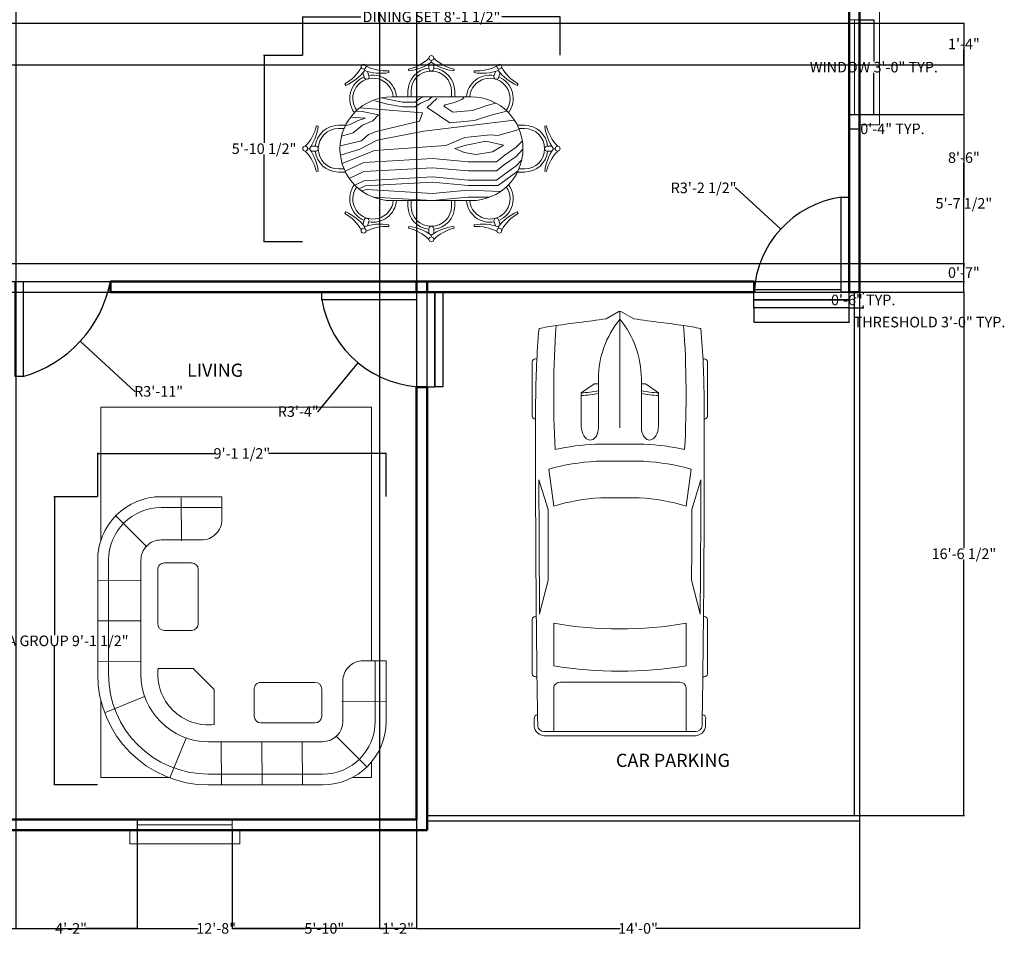
# Model space of a CAD drawing. Units: inches. Extents: x 749 to 1356, y 222 to 907.
# Tile 2 of 4: x 982 to 1356, y 222 to 570. Entities that reach past the tile are written whole.
import ezdxf

# ---------------------------------------------------------------- set-up
doc = ezdxf.new("R2010")
doc.units = ezdxf.units.IN
doc.header["$MEASUREMENT"] = 0
for name, color, linetype, lineweight in [('A-ANNO-DIMS', 30, 'Continuous', 18), ('A-AREA-IDEN', 6, 'Continuous', 25), ('A-EQPM-VEHI', 8, 'Continuous', 13), ('A-FLOR', 50, 'Continuous', 25), ('A-GLAZ', 4, 'Continuous', 20), ('A-WALL', 7, 'Continuous', 50), ('DOOR', 4, 'Continuous', 25), ('FURNITURE', 32, 'Continuous', 18)]:
    doc.layers.add(name, color=color, linetype=linetype, lineweight=lineweight)
doc.styles.get("Standard").update_dxf_attribs({"font": 'arial.ttf'})
doc.dimstyles.get("Standard").update_dxf_attribs({"dimtxt": 4, "dimasz": 0.18, "dimexe": 0.18, "dimexo": 0.0625, "dimgap": 0.09, "dimtad": 0, "dimtih": 1, "dimtoh": 1, "dimdec": 0, "dimrnd": 6, "dimzin": 0, "dimdsep": 46, "dimlunit": 3, "dimtxsty": 'Standard', "dimcen": 0.09, "dimadec": 0, "dimazin": 0, "dimtfac": 1, "dimtdec": 0, "dimtofl": 0, "dimtmove": 0, "dimatfit": 3, "dimfxl": 1, "dimtolj": 1, "dimtzin": 0, "dimarcsym": 0})

# ---------------------------------------------------------------- blocks, each defined once
blk = doc.blocks.new('ОГ56_на8персон_стол1760х1000')
for p, q in [((-54.1, 413.1), (-54.1, 412.2)), ((-713.5, 329), (-713.2, 328.1)), ((-77.6, 332.9), (-77.6, 291.9)), ((-54.1, 365), (-54.1, 348.6)), ((-30.5, 332.9), (-30.5, 291.9)), ((608.1, 329), (607.9, 328.1)), ((-713.2, 245.4), (-701.4, 206.1)), ((-699.7, 282.9), (-695.1, 267.2)), ((-668, 258.9), (-656.3, 219.5)), ((-464.6, 265.8), (-464.4, 247.7)), ((-274.5, 281.4), (-269.5, 264.1)), ((166.4, 281.4), (161.4, 264.1)), ((359.3, 265.8), (359.1, 247.7)), ((562.6, 258.9), (550.9, 219.5)), ((594.4, 282.9), (589.7, 267.2)), ((607.8, 245.4), (596.1, 206.1)), ((-887.1, 139.8), (-877.4, 124.6)), ((781.8, 139.8), (772.1, 124.6)), ((-279.1, 68.1), (-279.1, 15.3)), ((-279.1, 68.1), (-279.1, 15.3)), ((-249.1, 68.1), (-249.1, 14.5)), ((140.9, 68.1), (140.9, 14.5)), ((170.9, 68.1), (170.9, 15.3)), ((-1160.9, -264.3), (-1143.6, -269.2)), ((-947.6, -259.7), (-880.1, -259.7)), ((-126.6, -314.5), (745, -208.4)), ((842.3, -259.7), (774.8, -259.7)), ((842.3, -259.7), (774.8, -259.7)), ((1055.6, -264.3), (1038.2, -269.2)), ((-947.6, -289.7), (-894, -289.7)), ((-577.1, -401.6), (-126.6, -314.5)), ((842.3, -289.7), (788.7, -289.7)), ((-1212.4, -461.1), (-1171.4, -461.1)), ((-741, -488.6), (-577.1, -401.6)), ((1107.1, -461.1), (1066, -461.1)), ((-1292.6, -484.7), (-1291.7, -484.7)), ((-1244.5, -484.7), (-1228.1, -484.7)), ((-1212.4, -508.3), (-1171.4, -508.3)), ((-929.8, -546), (-741, -488.6)), ((1107.1, -508.3), (1066, -508.3)), ((1139.2, -484.7), (1122.8, -484.7)), ((1187.3, -484.7), (1186.3, -484.7)), ((-1160.9, -705.1), (-1143.6, -700.2)), ((-947.6, -679.7), (-894, -679.7)), ((-947.6, -709.7), (-880.1, -709.7)), ((842.3, -709.7), (774.8, -709.7)), ((842.3, -679.7), (788.7, -679.7)), ((1055.6, -705.1), (1038.2, -700.2)), ((-279.1, -1037.5), (-279.1, -984.7)), ((-279.1, -1037.5), (-279.1, -984.7)), ((-249.1, -1037.5), (-249.1, -983.9)), ((140.9, -1037.5), (140.9, -983.9)), ((170.9, -1037.5), (170.9, -984.7)), ((-887.1, -1109.2), (-877.4, -1094)), ((781.8, -1109.2), (772.1, -1094)), ((-713.2, -1214.8), (-701.4, -1175.5)), ((-668, -1228.3), (-656.3, -1188.9)), ((-464.6, -1235.1), (-464.4, -1217.1)), ((359.3, -1235.1), (359.1, -1217.1)), ((562.6, -1228.3), (550.9, -1188.9)), ((607.8, -1214.8), (596.1, -1175.5)), ((-713.5, -1298.4), (-713.2, -1297.5)), ((-699.7, -1252.3), (-695.1, -1236.6)), ((-274.5, -1250.8), (-269.5, -1233.5)), ((-77.6, -1302.3), (-77.6, -1261.3)), ((-54.1, -1334.4), (-54.1, -1318)), ((-30.5, -1302.3), (-30.5, -1261.3)), ((166.4, -1250.8), (161.4, -1233.5)), ((594.4, -1252.3), (589.7, -1236.6)), ((608.1, -1298.4), (607.9, -1297.5)), ((-54.1, -1382.5), (-54.1, -1381.6))]:
    blk.add_line(p, q)
for points in [[(-598.9, -24.3), (-476.4, -56.3), (-332.7, -82.9), (-210.2, -82.9), (-157, -45.6), (-82.5, -13.7), (-46.2, 15.3)], [(-530.7, 5.8), (-476.4, -8.4), (-332.7, -35), (-210.2, -35), (-157, 2.3), (-126.6, 15.3)], [(-433.6, 15.3), (328.3, 15.3)], [(672.4, -122), (509.9, -163.9), (362.7, -214.1), (125.3, -234.2), (-93.7, -88), (0, 0)], [(79.7, -62.3), (167.8, -40.3), (247.6, -8.4), (263.1, 15.3)], [(-932.9, -458.7), (-727.6, -408.3), (-657.4, -348), (-583.8, -317.9), (-166.7, -220.8), (-140, -140.5), (-743.6, -92.4)], [(567.6, -45.7), (481.2, -68), (342.1, -115.5), (151.7, -131.6), (66.5, -74.7), (79.7, -62.3)], [(-919.1, -365), (-807.9, -331.3), (-717.6, -257.6), (-617.2, -217.5), (-563.7, -157.2), (-720.9, -127.1), (-777.6, -121.8)], [(-883.3, -266.1), (-834.6, -252.1), (-757.7, -211.9), (-687.5, -191.8), (-830, -180)], [(793.2, -300.7), (587.2, -356.4), (515.4, -351.6), (268.7, -376.9), (85.4, -452.8), (-602.4, -503.4), (-913, -626.8)], [(822.3, -407.6), (762.6, -471.2), (653.6, -547.1), (573.6, -610.4), (301.7, -610.4), (-41.8, -578.8), (-702.3, -616.7), (-884.6, -700.6)], [(828.2, -490.2), (762.6, -560.1), (651.1, -636), (573.6, -699.3), (301.7, -699.3), (-41.8, -667.6), (-702.3, -705.6), (-843.8, -770.7)], [(816.8, -591.3), (762.6, -648.9), (658.7, -724.9), (573.6, -788.2), (301.7, -788.2), (-41.8, -756.5), (-702.3, -794.5), (-790.4, -835)], [(780.6, -697.7), (688.4, -765.1), (590.1, -838.2), (299.4, -838.2), (-42.7, -806.7), (-690, -843.9), (-750.3, -871.6)], [(609.5, -898.1), (296.3, -883.5), (-43.8, -914.8), (-673.5, -878.6), (-724.3, -891.5)], [(504.3, -952.7), (296.3, -952.7), (-43.8, -984), (-613.4, -951.3)], [(328.3, -984.7), (-433.6, -984.7)]]:
    blk.add_lwpolyline(points)
blk.add_lwpolyline([(641.8, -451.5), (534.3, -514.8), (376.2, -540.1), (262.4, -521.1), (173.9, -483.1), (281.4, -451.5), (471.1, -413.5)], close=True)
for centre in [(-54.1, 388.6), (-706.5, 305.5), (601.1, 305.5), (-1268.1, -484.7), (1162.8, -484.7), (-706.5, -1274.9), (601.1, -1274.9), (-54.1, -1358)]:
    blk.add_circle(centre, 23.6)
for centre, radius, start, end in [((-360.8, 674.3), 402.3, 282.38676, 314.74189), ((252.7, 674.3), 402.3, 225.25811, 257.61324), ((-1082, 491.8), 402.3, 298.97989, 331.33502), ((-494.1, 666.9), 402.3, 241.85124, 274.20637), ((-54.1, 68.1), 225, 96.01239, 180), ((-332.2, 740.5), 480.6, 277.49099, 305.35851), ((-54.1, 286.7), 23.6, 167.11156, 12.88844), ((224, 740.5), 480.6, 234.64149, 262.50901), ((-54.1, 68.1), 225, 0, 83.98761), ((388.8, 666.9), 402.3, 265.79363, 298.14876), ((976.7, 491.8), 402.3, 208.66498, 241.02011), ((-1073.5, 563.4), 480.6, 294.08412, 321.95164), ((-615, -1.6), 225, 112.60552, 217.31149), ((-615, -1.6), 195, 4.98125, 216.21895), ((-677.4, 207.8), 23.6, 183.7047, 29.48157), ((-540.5, 722.2), 480.6, 251.23462, 279.10214), ((-615, -1.6), 225, 4.31572, 100.58074), ((-54.1, 68.1), 195, 0, 180), ((509.6, -1.6), 225, 79.41926, 175.68428), ((509.6, -1.6), 195, 323.78105, 175.01875), ((435.1, 722.2), 480.6, 260.89786, 288.76538), ((572, 207.8), 23.6, 150.51843, 356.2953), ((968.2, 563.4), 480.6, 218.04836, 245.91588), ((509.6, -1.6), 225, 322.68851, 67.39448), ((-433.6, -484.7), 500, 90, 270), ((328.3, -484.7), 500, 270, 90), ((-1553.8, -178), 402.3, 315.25811, 347.61324), ((-1620, -206.6), 480.6, 324.64149, 352.50901), ((-947.6, -484.7), 225, 90, 173.98761), ((842.3, -484.7), 225, 6.01239, 90), ((1514.7, -206.6), 480.6, 187.49099, 215.35851), ((1448.5, -178), 402.3, 192.38676, 224.74189), ((-947.6, -484.7), 195, 90, 270), ((842.3, -484.7), 195, 270, 90), ((-1166.2, -484.7), 23.6, 257.11156, 102.88844), ((1060.8, -484.7), 23.6, 77.11156, 282.88844), ((-1553.8, -791.4), 402.3, 12.38676, 44.74189), ((-1620, -762.8), 480.6, 7.49099, 35.35851), ((-947.6, -484.7), 225, 186.01239, 270), ((842.3, -484.7), 225, 270, 353.98761), ((1514.7, -762.8), 480.6, 144.64149, 172.50901), ((1448.5, -791.4), 402.3, 135.25811, 167.61324), ((-615, -967.8), 225, 142.68851, 247.39448), ((-615, -967.8), 195, 143.78105, 355.01875), ((509.6, -967.8), 195, 184.98125, 36.21895), ((509.6, -967.8), 225, 292.60552, 37.31149), ((-615, -967.8), 225, 259.41926, 355.68428), ((-54.1, -1037.5), 225, 180, 263.98761), ((-54.1, -1037.5), 195, 180, 0), ((-54.1, -1037.5), 225, 276.01239, 0), ((509.6, -967.8), 225, 184.31572, 280.58074), ((-1082, -1461.1), 402.3, 28.66498, 61.02011), ((-1073.5, -1532.8), 480.6, 38.04836, 65.91588), ((968.2, -1532.8), 480.6, 114.08412, 141.95164), ((976.7, -1461.1), 402.3, 118.97989, 151.33502), ((-677.4, -1177.2), 23.6, 330.51843, 176.2953), ((-540.5, -1691.6), 480.6, 80.89786, 108.76538), ((435.1, -1691.6), 480.6, 71.23462, 99.10214), ((572, -1177.2), 23.6, 3.7047, 209.48157), ((-494.1, -1636.3), 402.3, 85.79363, 118.14876), ((-360.8, -1643.7), 402.3, 45.25811, 77.61324), ((-332.2, -1709.9), 480.6, 54.64149, 82.50901), ((-54.1, -1256.1), 23.6, 347.11156, 192.88844), ((224, -1709.9), 480.6, 97.49099, 125.35851), ((252.7, -1643.7), 402.3, 102.38676, 134.74189), ((388.8, -1636.3), 402.3, 61.85124, 94.20637)]:
    blk.add_arc(centre, radius, start, end)
blk = doc.blocks.new('A$C0BCD5431')
for p, q in [((2628, 4268), (940, 4268)), ((1236, 4268), (1240, 3628)), ((1836, 4268), (1840, 3628)), ((2436, 4268), (2440, 3628)), ((2628, 4108), (940, 4108)), ((2957, 3573), (3201, 4165)), ((742, 3540), (290, 3993)), ((2628, 3628), (940, 3628)), ((2542, 3373), (2545, 2855)), ((0, 3328), (0, 2432)), ((160, 3328), (160, 2431)), ((640, 3328), (640, 2730)), ((952, 3249), (952, 2849)), ((1852, 3349), (1052, 3349)), ((1952, 2849), (1952, 3249)), ((3573, 2957), (4165, 3201)), ((15, 3032), (655, 3028)), ((2545, 2855), (2855, 2545)), ((1052, 2749), (1852, 2749)), ((3628, 2628), (3628, 940)), ((4108, 2628), (4108, 940)), ((4268, 2628), (4268, 940)), ((3373, 2542), (2855, 2545)), ((0, 2432), (338, 2430)), ((4268, 2436), (3628, 2440)), ((3280, 1980), (2880, 1980)), ((2780, 1880), (2780, 1080)), ((3380, 1080), (3380, 1880)), ((4268, 1836), (3628, 1840)), ((4268, 1236), (3628, 1240)), ((2880, 980), (3280, 980)), ((3540, 742), (3993, 290)), ((3328, 640), (2730, 640)), ((3032, 15), (3028, 655)), ((2432, 0), (2430, 338)), ((3328, 160), (2431, 160)), ((3328, 0), (2432, 0))]:
    blk.add_line(p, q)
for centre, radius, start, end in [((940, 3328), 940, 90, 180), ((2628, 2628), 1640, 0, 90), ((940, 3328), 780, 90, 180), ((2628, 2628), 1480, 0, 90), ((940, 3328), 300, 90, 180), ((2628, 2628), 1000, 0, 90), ((2628, 2628), 750, 353.3601, 96.6399), ((1052, 3249), 100, 90, 180), ((1852, 3249), 100, 0, 90), ((1052, 2849), 100, 180, 270), ((1852, 2849), 100, 270, 0), ((340, 2730), 300, 269.6481, 0), ((2880, 1880), 100, 90, 180), ((3280, 1880), 100, 0, 90), ((2880, 1080), 100, 180, 270), ((3280, 1080), 100, 270, 0), ((3328, 940), 300, 270, 0), ((3328, 940), 780, 270, 0), ((3328, 940), 940, 270, 0), ((2730, 340), 300, 90, 180.3519)]:
    blk.add_arc(centre, radius, start, end)
blk = doc.blocks.new('*U128')
for p, q in [((21.1, 37.41), (21.1, 36.83)), ((46.55, 38.89), (22.35, 38.89)), ((47.8, 37.39), (47.8, 37.41)), ((87.99, 31.87), (74.76, 35.92)), ((134.31, 35.6), (119.29, 31.78)), ((135.45, 37.07), (135.45, 37.41)), ((136.7, 38.89), (160.9, 38.89)), ((162.15, 37.41), (162.15, 36.77)), ((70.03, 31.54), (86.41, 29.35)), ((186.47, -33.5), (186.47, 33.5)), ((188.4, -32.76), (188.4, 32.76)), ((138.42, 29.35), (157.25, 29.35)), ((164.52, 26.39), (164.52, -26.39)), ((186.47, 29.35), (167.01, 29.35)), ((32.27, 11.63), (36.13, 17.17)), ((36.13, 17.17), (50.94, 17.17)), ((29.77, 9.51), (51.68, 9.51)), ((32.12, 9.51), (32.12, 11.15)), ((58.92, -10.77), (58.92, 10.77)), ((66.55, -10.53), (66.55, 10.53)), ((186.47, -10.53), (186.47, 10.53)), ((3.27, 6.13), (0.1, 0.41)), ((82.74, 8.5), (82.74, -8.5)), ((0, 0), (51.68, 0)), ((0.1, -0.41), (3.27, -6.13)), ((29.77, -9.51), (51.68, -9.51)), ((32.12, -9.51), (32.12, -11.15)), ((32.27, -11.63), (36.13, -17.17)), ((36.13, -17.17), (50.94, -17.17)), ((86.41, -29.35), (70.03, -31.54)), ((157.25, -29.35), (138.42, -29.35)), ((167.01, -29.35), (186.47, -29.35)), ((87.99, -31.87), (74.76, -35.92)), ((134.31, -35.6), (119.29, -31.78)), ((21.1, -37.41), (21.1, -36.83)), ((46.55, -38.89), (22.35, -38.89)), ((47.8, -37.39), (47.8, -37.41)), ((135.45, -37.07), (135.45, -37.41)), ((136.7, -38.89), (160.9, -38.89)), ((162.15, -37.41), (162.15, -36.77))]:
    blk.add_line(p, q)
for centre, major_axis, ratio, start_param, end_param in [((266.03, -27.52), (0, 313.31), 0.842304, 1.367076, 1.39176), ((41.19, -490.86), (0, 528.23), 0.842304, 0.00281, 0.075598), ((22.35, 37.41), (0, -1.48), 0.842304, 3.141593, 4.712389), ((64.48, -10555.62), (0, 10593.03), 0.842304, -0.013397, 0.002797), ((46.55, 37.41), (0, 1.48), 0.842304, -1.570796, 0), ((64.48, -10555.62), (0, -10591.55), 0.842304, 3.133765, 3.140441), ((136.7, 37.41), (0, -1.48), 0.842304, 3.141593, 4.712389), ((160.9, 37.41), (0, 1.48), 0.842304, -1.570796, 0), ((180.63, 35.84), (0, 2.22), 0.842304, -0.013017, 1.249894), ((64.48, -10556.36), (0, 10595.31), 0.842304, -0.013397, -0.013017), ((183.98, 33.5), (0, -2.96), 0.842304, 1.570796, 3.128196), ((183.98, 32.76), (0, -5.25), 0.842304, 1.570796, 3.128196), ((135.29, 5.39), (0, 81.77), 0.842304, 1.245306, 1.50788), ((95.79, -3666.35), (0, -3698.24), 0.842304, 3.134049, 3.144098), ((259.18, -27.52), (0, -305.3), 0.842304, 4.528606, 4.561838), ((37.47, -593.96), (0, -623.33), 0.842304, 3.096046, 3.200911), ((134.4, 5.39), (0, -89.78), 0.842304, 4.449482, 4.652344), ((149.6, 2.8), (0, -79.58), 0.842304, 4.372215, 4.640744), ((17.08, 0), (0, 147.02), 0.842304, 4.511394, 4.913384), ((35.91, 0), (0, 147.02), 0.842304, 4.511394, 4.913384), ((167.01, 26.39), (0, 2.96), 0.842304, 0, 1.570796), ((-204.49, 52.4), (0, -250.96), 0.842304, 1.385369, 1.434372), ((13.04, 17.01), (0, 27.42), 0.842304, 4.435146, 4.718221), ((14.2, 17.01), (0, 27.42), 0.842304, 4.435146, 4.718221), ((50.79, 13.34), (6.34, -0.36), 0.603834, -1.395552, 1.581315), ((29.77, -46.66), (0, 56.17), 0.842304, 0, 0.590319), ((32.75, 11.15), (0, 0.74), 0.842304, 0.879714, 1.570796), ((0.62, 0), (0, -0.74), 0.842304, 4.131459, 5.293319), ((29.77, 46.66), (0, 56.17), 0.842304, 2.551274, 3.141593), ((-204.49, -52.4), (0, 250.96), 0.842304, -1.434372, -1.385369), ((149.6, -2.8), (0, -79.58), 0.842304, -1.499151, -1.230623), ((32.75, -11.15), (0, -0.74), 0.842304, 4.712389, 5.403472), ((13.04, -17.01), (0, -27.42), 0.842304, 1.564964, 1.848039), ((14.2, -17.01), (0, -27.42), 0.842304, 1.564964, 1.848039), ((134.4, -5.39), (0, -89.78), 0.842304, -1.510751, -1.307889), ((135.29, -5.39), (0, -81.77), 0.842304, -1.50788, -1.245306), ((259.18, 27.52), (0, 305.3), 0.842304, 1.721348, 1.754579), ((266.03, 27.52), (0, 313.31), 0.842304, 1.749832, 1.774517), ((37.47, 593.96), (0, -623.33), 0.842304, -0.059319, 0.045547), ((167.01, -26.39), (0, -2.96), 0.842304, 4.712389, 6.283185), ((95.79, 3666.35), (0, -3698.24), 0.842304, -0.002505, 0.007544), ((183.98, -33.5), (0, 2.96), 0.842304, 3.15499, 4.712389), ((183.98, -32.76), (0, -5.25), 0.842304, 0.013397, 1.570796), ((41.19, 490.86), (0, -528.23), 0.842304, -0.075598, -0.00281), ((22.35, -37.41), (0, 1.48), 0.842304, 1.570796, 3.141593), ((64.48, 10555.62), (0, 10593.03), 0.842304, 3.138796, 3.15499), ((46.55, -37.41), (0, -1.48), 0.842304, 0, 1.570796), ((64.48, 10555.62), (0, -10591.55), 0.842304, 0.001152, 0.007828), ((136.7, -37.41), (0, -1.48), 0.842304, -1.570796, 0), ((160.9, -37.41), (0, 1.48), 0.842304, 3.141593, 4.712389), ((180.63, -35.84), (0, -2.22), 0.842304, -1.249894, 0.013017), ((64.48, 10556.36), (0, 10595.31), 0.842304, 3.15461, 3.15499)]:
    blk.add_ellipse(centre, major_axis=major_axis, ratio=ratio, start_param=start_param, end_param=end_param)
at = {"extrusion": (0, 0, -1)}
blk.add_ellipse((50.79, -13.34), major_axis=(6.34, 0.36), ratio=0.603834, start_param=-1.395552, end_param=1.581315, dxfattribs=at)
blk = doc.blocks.new('WIN-36IN')
blk.add_lwpolyline([(0, 0), (0, 36), (4, 36), (4, 0)], close=True)
blk.add_lwpolyline([(4, 0), (2.02, 0), (2.02, 36)])
blk = doc.blocks.new('DOOR-THRESHOLD-36IN')
for points in [[(0, 6), (36, 6), (36, 3), (0, 3)], [(0.01, 3), (36.01, 3), (36.01, 0), (0.01, 0)]]:
    blk.add_lwpolyline(points, close=True)
blk = doc.blocks.new('DOOR-LEAF-36IN')
blk.add_lwpolyline([(0, 3), (36, 3), (36, 0), (0, 0)], close=True)
blk = doc.blocks.new('*D135')
at = {"layer": 'A-ANNO-DIMS', "color": 0, "lineweight": -2, "transparency": 16777216}
for p, q in [((1300.93, 569.57), (1306.45, 569.57)), ((1306.27, 569.39), (1306.27, 553.73)), ((1306.27, 533.75), (1306.27, 549.41)), ((1300.93, 533.57), (1306.45, 533.57))]:
    blk.add_line(p, q, dxfattribs=at)
at = {"layer": 'A-ANNO-DIMS', "color": 0, "transparency": 16777216}
for points in [[(1306.24, 569.39), (1306.3, 569.39), (1306.27, 569.57)], [(1306.24, 533.75), (1306.3, 533.75), (1306.27, 533.57)]]:
    blk.add_solid(points, dxfattribs=at)
at = {"layer": 'Defpoints', "color": 0, "transparency": 16777216}
for p in [(1300.87, 569.57), (1306.27, 569.57), (1300.87, 533.57)]:
    blk.add_point(p, dxfattribs=at)
at = {"layer": 'A-ANNO-DIMS', "color": 0, "transparency": 16777216, "insert": (1306.27, 551.57), "char_height": 4, "attachment_point": 5}
blk.add_mtext('\\A1;WINDOW 3\'-0" TYP.', dxfattribs=at)
blk = doc.blocks.new('*D136')
at = {"layer": 'A-ANNO-DIMS', "color": 0, "lineweight": -2, "transparency": 16777216}
for p, q in [((1296.87, 533.5), (1296.87, 527.99)), ((1300.87, 533.5), (1300.87, 527.99)), ((1297.05, 528.17), (1300.69, 528.17)), ((1300.87, 528.17), (1301.05, 528.17))]:
    blk.add_line(p, q, dxfattribs=at)
at = {"layer": 'A-ANNO-DIMS', "color": 0, "transparency": 16777216}
for points in [[(1297.05, 528.2), (1297.05, 528.14), (1296.87, 528.17)], [(1300.69, 528.2), (1300.69, 528.14), (1300.87, 528.17)]]:
    blk.add_solid(points, dxfattribs=at)
at = {"layer": 'Defpoints', "color": 0, "transparency": 16777216}
for p in [(1296.87, 533.57), (1300.87, 533.57), (1300.87, 528.17)]:
    blk.add_point(p, dxfattribs=at)
at = {"layer": 'A-ANNO-DIMS', "color": 0, "transparency": 16777216, "insert": (1313.33, 528.17), "char_height": 4, "attachment_point": 5}
blk.add_mtext('\\A1;0\'-4" TYP.', dxfattribs=at)
blk = doc.blocks.new('*D139')
at = {"layer": 'A-ANNO-DIMS', "color": 0, "lineweight": -2, "transparency": 16777216}
for p, q in [((1260.82, 460.23), (1260.82, 454.71)), ((1296.83, 460.23), (1296.83, 454.71)), ((1261, 454.89), (1296.65, 454.89)), ((1296.83, 454.89), (1297.01, 454.89))]:
    blk.add_line(p, q, dxfattribs=at)
at = {"layer": 'A-ANNO-DIMS', "color": 0, "transparency": 16777216}
for points in [[(1261, 454.92), (1261, 454.86), (1260.82, 454.89)], [(1296.65, 454.92), (1296.65, 454.86), (1296.83, 454.89)]]:
    blk.add_solid(points, dxfattribs=at)
at = {"layer": 'Defpoints', "color": 0, "transparency": 16777216}
for p in [(1260.82, 460.29), (1296.83, 460.29), (1296.83, 454.89)]:
    blk.add_point(p, dxfattribs=at)
at = {"layer": 'A-ANNO-DIMS', "color": 0, "transparency": 16777216, "insert": (1327.35, 454.89), "char_height": 4, "attachment_point": 5}
blk.add_mtext('\\A1;THRESHOLD 3\'-0" TYP.', dxfattribs=at)
blk = doc.blocks.new('*D140')
at = {"layer": 'A-ANNO-DIMS', "color": 0, "lineweight": -2, "transparency": 16777216}
for p, q in [((1296.89, 466.29), (1302.41, 466.29)), ((1302.23, 466.11), (1302.23, 465.43)), ((1296.89, 460.29), (1302.41, 460.29)), ((1302.23, 460.47), (1302.23, 461.16))]:
    blk.add_line(p, q, dxfattribs=at)
at = {"layer": 'A-ANNO-DIMS', "color": 0, "transparency": 16777216}
for points in [[(1302.2, 466.11), (1302.26, 466.11), (1302.23, 466.29)], [(1302.2, 460.47), (1302.26, 460.47), (1302.23, 460.29)]]:
    blk.add_solid(points, dxfattribs=at)
at = {"layer": 'Defpoints', "color": 0, "transparency": 16777216}
for p in [(1296.83, 466.29), (1302.23, 466.29), (1296.83, 460.29)]:
    blk.add_point(p, dxfattribs=at)
at = {"layer": 'A-ANNO-DIMS', "color": 0, "transparency": 16777216, "insert": (1302.23, 463.29), "char_height": 4, "attachment_point": 5}
blk.add_mtext('\\A1;0\'-6" TYP.', dxfattribs=at)
blk = doc.blocks.new('*D151')
at = {"layer": 'A-ANNO-DIMS', "color": 0, "lineweight": -2, "transparency": 16777216}
for p, q in [((1089.75, 556.06), (1089.75, 570.82)), ((1089.93, 570.64), (1111.83, 570.64)), ((1187.2, 570.64), (1165.29, 570.64)), ((1187.38, 556.06), (1187.38, 570.82))]:
    blk.add_line(p, q, dxfattribs=at)
at = {"layer": 'A-ANNO-DIMS', "color": 0, "transparency": 16777216}
for points in [[(1089.93, 570.67), (1089.93, 570.61), (1089.75, 570.64)], [(1187.2, 570.67), (1187.2, 570.61), (1187.38, 570.64)]]:
    blk.add_solid(points, dxfattribs=at)
at = {"layer": 'Defpoints', "color": 0, "transparency": 16777216}
for p in [(1187.38, 570.64), (1089.75, 556), (1187.38, 556)]:
    blk.add_point(p, dxfattribs=at)
at = {"layer": 'A-ANNO-DIMS', "color": 0, "transparency": 16777216, "insert": (1138.56, 570.64), "char_height": 4, "attachment_point": 5}
blk.add_mtext('\\A1;DINING SET 8\'-1 1/2"', dxfattribs=at)
blk = doc.blocks.new('*D152')
at = {"layer": 'A-ANNO-DIMS', "color": 0, "lineweight": -2, "transparency": 16777216}
for p, q in [((1089.68, 556), (1074.92, 556)), ((1075.1, 555.82), (1075.1, 522.81)), ((1075.1, 485.48), (1075.1, 518.49)), ((1089.68, 485.3), (1074.92, 485.3))]:
    blk.add_line(p, q, dxfattribs=at)
at = {"layer": 'A-ANNO-DIMS', "color": 0, "transparency": 16777216}
for points in [[(1075.07, 555.82), (1075.13, 555.82), (1075.1, 556)], [(1075.07, 485.48), (1075.13, 485.48), (1075.1, 485.3)]]:
    blk.add_solid(points, dxfattribs=at)
at = {"layer": 'Defpoints', "color": 0, "transparency": 16777216}
for p in [(1075.1, 556), (1089.75, 556), (1089.75, 485.3)]:
    blk.add_point(p, dxfattribs=at)
at = {"layer": 'A-ANNO-DIMS', "color": 0, "transparency": 16777216, "insert": (1075.1, 520.65), "char_height": 4, "attachment_point": 5}
blk.add_mtext('\\A1;5\'-10 1/2"', dxfattribs=at)
blk = doc.blocks.new('*D153')
at = {"layer": 'A-ANNO-DIMS', "color": 0, "lineweight": -2, "transparency": 16777216}
for p, q in [((1011.97, 388.69), (995.45, 388.69)), ((995.63, 388.51), (995.63, 336.18)), ((995.63, 279.54), (995.63, 331.87)), ((1011.97, 279.36), (995.45, 279.36))]:
    blk.add_line(p, q, dxfattribs=at)
at = {"layer": 'A-ANNO-DIMS', "color": 0, "transparency": 16777216}
for points in [[(995.6, 388.51), (995.66, 388.51), (995.63, 388.69)], [(995.6, 279.54), (995.66, 279.54), (995.63, 279.36)]]:
    blk.add_solid(points, dxfattribs=at)
at = {"layer": 'Defpoints', "color": 0, "transparency": 16777216}
for p in [(1012.03, 388.69), (995.63, 279.36), (1012.03, 279.36)]:
    blk.add_point(p, dxfattribs=at)
at = {"layer": 'A-ANNO-DIMS', "color": 0, "transparency": 16777216, "insert": (995.63, 334.02), "char_height": 4, "attachment_point": 5}
blk.add_mtext('\\A1;SOFA GROUP 9\'-1 1/2"', dxfattribs=at)
blk = doc.blocks.new('*D154')
at = {"layer": 'A-ANNO-DIMS', "color": 0, "lineweight": -2, "transparency": 16777216}
for p, q in [((1012.03, 388.75), (1012.03, 405.26)), ((1012.21, 405.08), (1056.63, 405.08)), ((1121.17, 405.08), (1076.76, 405.08)), ((1121.35, 388.75), (1121.35, 405.26))]:
    blk.add_line(p, q, dxfattribs=at)
at = {"layer": 'A-ANNO-DIMS', "color": 0, "transparency": 16777216}
for points in [[(1012.21, 405.11), (1012.21, 405.05), (1012.03, 405.08)], [(1121.17, 405.11), (1121.17, 405.05), (1121.35, 405.08)]]:
    blk.add_solid(points, dxfattribs=at)
at = {"layer": 'Defpoints', "color": 0, "transparency": 16777216}
for p in [(1012.03, 405.08), (1012.03, 388.69), (1121.35, 388.69)]:
    blk.add_point(p, dxfattribs=at)
at = {"layer": 'A-ANNO-DIMS', "color": 0, "transparency": 16777216, "insert": (1066.69, 405.08), "char_height": 4, "attachment_point": 5}
blk.add_mtext('\\A1;9\'-1 1/2"', dxfattribs=at)
blk = doc.blocks.new('*D156')
at = {"layer": 'A-ANNO-DIMS', "color": 0, "lineweight": -2, "transparency": 16777216}
for p, q in [((976.88, 266.2), (976.88, 224.8)), ((1027.01, 266.19), (1027.01, 224.8)), ((977.06, 224.98), (996.46, 224.98)), ((1026.83, 224.98), (1007.43, 224.98))]:
    blk.add_line(p, q, dxfattribs=at)
at = {"layer": 'A-ANNO-DIMS', "color": 0, "transparency": 16777216}
for points in [[(977.06, 225.01), (977.06, 224.95), (976.88, 224.98)], [(1026.83, 225.01), (1026.83, 224.95), (1027.01, 224.98)]]:
    blk.add_solid(points, dxfattribs=at)
at = {"layer": 'Defpoints', "color": 0, "transparency": 16777216}
for p in [(976.88, 266.27), (1027.01, 266.25), (1027.01, 224.98)]:
    blk.add_point(p, dxfattribs=at)
at = {"layer": 'A-ANNO-DIMS', "color": 0, "transparency": 16777216, "insert": (1001.95, 224.98), "char_height": 4, "attachment_point": 5}
blk.add_mtext('\\A1;4\'-2"', dxfattribs=at)
blk = doc.blocks.new('*D157')
at = {"layer": 'A-ANNO-DIMS', "color": 0, "lineweight": -2, "transparency": 16777216}
for p, q in [((1132.88, 266.2), (1132.88, 224.8)), ((1063.01, 262.19), (1063.01, 224.8)), ((1063.19, 224.98), (1090.98, 224.98)), ((1132.7, 224.98), (1104.91, 224.98))]:
    blk.add_line(p, q, dxfattribs=at)
at = {"layer": 'A-ANNO-DIMS', "color": 0, "transparency": 16777216}
for points in [[(1063.19, 225.01), (1063.19, 224.95), (1063.01, 224.98)], [(1132.7, 225.01), (1132.7, 224.95), (1132.88, 224.98)]]:
    blk.add_solid(points, dxfattribs=at)
at = {"layer": 'Defpoints', "color": 0, "transparency": 16777216}
for p in [(1132.88, 266.27), (1063.01, 262.25), (1132.88, 224.98)]:
    blk.add_point(p, dxfattribs=at)
at = {"layer": 'A-ANNO-DIMS', "color": 0, "transparency": 16777216, "insert": (1097.95, 224.98), "char_height": 4, "attachment_point": 5}
blk.add_mtext('\\A1;5\'-10"', dxfattribs=at)
blk = doc.blocks.new('*D158')
at = {"layer": 'A-ANNO-DIMS', "color": 0, "lineweight": -2, "transparency": 16777216}
for p, q in [((1132.88, 266.2), (1132.88, 224.8)), ((1300.84, 265.75), (1300.84, 224.8)), ((1133.06, 224.98), (1210.09, 224.98)), ((1300.66, 224.98), (1223.63, 224.98))]:
    blk.add_line(p, q, dxfattribs=at)
at = {"layer": 'A-ANNO-DIMS', "color": 0, "transparency": 16777216}
for points in [[(1133.06, 225.01), (1133.06, 224.95), (1132.88, 224.98)], [(1300.66, 225.01), (1300.66, 224.95), (1300.84, 224.98)]]:
    blk.add_solid(points, dxfattribs=at)
at = {"layer": 'Defpoints', "color": 0, "transparency": 16777216}
for p in [(1132.88, 266.27), (1300.84, 265.82), (1300.84, 224.98)]:
    blk.add_point(p, dxfattribs=at)
at = {"layer": 'A-ANNO-DIMS', "color": 0, "transparency": 16777216, "insert": (1216.86, 224.98), "char_height": 4, "attachment_point": 5}
blk.add_mtext('\\A1;14\'-0"', dxfattribs=at)
blk = doc.blocks.new('*D162')
at = {"layer": 'A-ANNO-DIMS', "color": 0, "lineweight": -2, "transparency": 16777216}
for p, q in [((1296.93, 533.57), (1340.58, 533.57)), ((1340.4, 533.39), (1340.4, 502.07)), ((1340.4, 466.45), (1340.4, 497.76)), ((1300.94, 466.27), (1340.58, 466.27))]:
    blk.add_line(p, q, dxfattribs=at)
at = {"layer": 'A-ANNO-DIMS', "color": 0, "transparency": 16777216}
for points in [[(1340.37, 533.39), (1340.43, 533.39), (1340.4, 533.57)], [(1340.37, 466.45), (1340.43, 466.45), (1340.4, 466.27)]]:
    blk.add_solid(points, dxfattribs=at)
at = {"layer": 'Defpoints', "color": 0, "transparency": 16777216}
for p in [(1296.87, 533.57), (1340.4, 533.57), (1300.88, 466.27)]:
    blk.add_point(p, dxfattribs=at)
at = {"layer": 'A-ANNO-DIMS', "color": 0, "transparency": 16777216, "insert": (1340.4, 499.92), "char_height": 4, "attachment_point": 5}
blk.add_mtext('\\A1;5\'-7 1/2"', dxfattribs=at)
blk = doc.blocks.new('*D168')
at = {"layer": 'A-ANNO-DIMS', "color": 0, "lineweight": -2, "transparency": 16777216}
for p, q in [((1296.94, 466.27), (1340.58, 466.27)), ((1340.4, 466.09), (1340.4, 369.2)), ((1340.4, 268), (1340.4, 364.88)), ((1298.9, 267.82), (1340.58, 267.82))]:
    blk.add_line(p, q, dxfattribs=at)
at = {"layer": 'A-ANNO-DIMS', "color": 0, "transparency": 16777216}
for points in [[(1340.37, 466.09), (1340.43, 466.09), (1340.4, 466.27)], [(1340.37, 268), (1340.43, 268), (1340.4, 267.82)]]:
    blk.add_solid(points, dxfattribs=at)
at = {"layer": 'Defpoints', "color": 0, "transparency": 16777216}
for p in [(1296.88, 466.27), (1340.4, 466.27), (1298.84, 267.82)]:
    blk.add_point(p, dxfattribs=at)
at = {"layer": 'A-ANNO-DIMS', "color": 0, "transparency": 16777216, "insert": (1340.4, 367.04), "char_height": 4, "attachment_point": 5}
blk.add_mtext('\\A1;16\'-6 1/2"', dxfattribs=at)
blk = doc.blocks.new('*D173')
at = {"layer": 'A-ANNO-DIMS', "color": 0, "lineweight": -2, "transparency": 16777216}
for p, q in [((896.94, 568.27), (1340.58, 568.27)), ((1340.4, 568.09), (1340.4, 519.4)), ((1340.4, 466.45), (1340.4, 515.13)), ((900.94, 466.27), (1340.58, 466.27))]:
    blk.add_line(p, q, dxfattribs=at)
at = {"layer": 'A-ANNO-DIMS', "color": 0, "transparency": 16777216}
for points in [[(1340.37, 568.09), (1340.43, 568.09), (1340.4, 568.27)], [(1340.37, 466.45), (1340.43, 466.45), (1340.4, 466.27)]]:
    blk.add_solid(points, dxfattribs=at)
at = {"layer": 'Defpoints', "color": 0, "transparency": 16777216}
for p in [(896.88, 568.27), (1340.4, 568.27), (900.88, 466.27)]:
    blk.add_point(p, dxfattribs=at)
at = {"layer": 'A-ANNO-DIMS', "color": 0, "transparency": 16777216, "insert": (1340.4, 517.27), "char_height": 4, "attachment_point": 5}
blk.add_mtext('\\A1;8\'-6"', dxfattribs=at)
blk = doc.blocks.new('*D180')
at = {"layer": 'A-ANNO-DIMS', "color": 0, "lineweight": -2, "transparency": 16777216}
for p, q in [((980.98, 762.26), (980.98, 224.8)), ((1132.88, 762.2), (1132.88, 224.8)), ((981.16, 224.98), (1050.16, 224.98)), ((1132.7, 224.98), (1063.7, 224.98))]:
    blk.add_line(p, q, dxfattribs=at)
at = {"layer": 'A-ANNO-DIMS', "color": 0, "transparency": 16777216}
for points in [[(981.16, 225.01), (981.16, 224.95), (980.98, 224.98)], [(1132.7, 225.01), (1132.7, 224.95), (1132.88, 224.98)]]:
    blk.add_solid(points, dxfattribs=at)
at = {"layer": 'Defpoints', "color": 0, "transparency": 16777216}
for p in [(980.98, 762.32), (1132.88, 762.27), (1132.88, 224.98)]:
    blk.add_point(p, dxfattribs=at)
at = {"layer": 'A-ANNO-DIMS', "color": 0, "transparency": 16777216, "insert": (1056.93, 224.98), "char_height": 4, "attachment_point": 5}
blk.add_mtext('\\A1;12\'-8"', dxfattribs=at)
blk = doc.blocks.new('*D185')
at = {"layer": 'A-ANNO-DIMS', "color": 0, "lineweight": -2, "transparency": 16777216}
for p, q in [((1132.88, 858.2), (1132.88, 224.8)), ((1118.88, 843.77), (1118.88, 224.8)), ((1119.06, 224.98), (1120.66, 224.98)), ((1132.7, 224.98), (1131.1, 224.98))]:
    blk.add_line(p, q, dxfattribs=at)
at = {"layer": 'A-ANNO-DIMS', "color": 0, "transparency": 16777216}
for points in [[(1119.06, 225.01), (1119.06, 224.95), (1118.88, 224.98)], [(1132.7, 225.01), (1132.7, 224.95), (1132.88, 224.98)]]:
    blk.add_solid(points, dxfattribs=at)
at = {"layer": 'Defpoints', "color": 0, "transparency": 16777216}
for p in [(1132.88, 858.27), (1118.88, 843.83), (1132.88, 224.98)]:
    blk.add_point(p, dxfattribs=at)
at = {"layer": 'A-ANNO-DIMS', "color": 0, "transparency": 16777216, "insert": (1125.88, 224.98), "char_height": 4, "attachment_point": 5}
blk.add_mtext('\\A1;1\'-2"', dxfattribs=at)
blk = doc.blocks.new('*D189')
at = {"layer": 'A-ANNO-DIMS', "color": 0, "lineweight": -2, "transparency": 16777216}
for p, q in [((829.64, 477.07), (1340.58, 477.07)), ((1340.4, 476.89), (1340.4, 475.8)), ((1340.4, 470.45), (1340.4, 471.54)), ((824.94, 470.27), (1340.58, 470.27))]:
    blk.add_line(p, q, dxfattribs=at)
at = {"layer": 'A-ANNO-DIMS', "color": 0, "transparency": 16777216}
for points in [[(1340.37, 476.89), (1340.43, 476.89), (1340.4, 477.07)], [(1340.37, 470.45), (1340.43, 470.45), (1340.4, 470.27)]]:
    blk.add_solid(points, dxfattribs=at)
at = {"layer": 'Defpoints', "color": 0, "transparency": 16777216}
for p in [(829.57, 477.07), (824.88, 470.27), (1340.4, 470.27)]:
    blk.add_point(p, dxfattribs=at)
at = {"layer": 'A-ANNO-DIMS', "color": 0, "transparency": 16777216, "insert": (1340.4, 473.67), "char_height": 4, "attachment_point": 5}
blk.add_mtext('\\A1;0\'-7"', dxfattribs=at)
blk = doc.blocks.new('*D190')
at = {"layer": 'A-ANNO-DIMS', "color": 0, "lineweight": -2, "transparency": 16777216}
for p, q in [((824.94, 568.27), (1340.58, 568.27)), ((1340.4, 568.09), (1340.4, 562.47)), ((1340.4, 552.65), (1340.4, 558.27)), ((828.78, 552.47), (1340.58, 552.47))]:
    blk.add_line(p, q, dxfattribs=at)
at = {"layer": 'A-ANNO-DIMS', "color": 0, "transparency": 16777216}
for points in [[(1340.37, 568.09), (1340.43, 568.09), (1340.4, 568.27)], [(1340.37, 552.65), (1340.43, 552.65), (1340.4, 552.47)]]:
    blk.add_solid(points, dxfattribs=at)
at = {"layer": 'Defpoints', "color": 0, "transparency": 16777216}
for p in [(824.88, 568.27), (1340.4, 568.27), (828.71, 552.47)]:
    blk.add_point(p, dxfattribs=at)
at = {"layer": 'A-ANNO-DIMS', "color": 0, "transparency": 16777216, "insert": (1340.4, 560.37), "char_height": 4, "attachment_point": 5}
blk.add_mtext('\\A1;1\'-4"', dxfattribs=at)
blk = doc.blocks.new('*D191')
at = {"layer": 'A-ANNO-DIMS', "color": 0, "lineweight": -2, "transparency": 16777216}
for p, q in [((970.9, 479.27), (971.08, 479.27)), ((970.99, 479.18), (970.99, 479.36)), ((1026.07, 428.63), (1005.55, 447.5)), ((1026.25, 428.63), (1026.07, 428.63))]:
    blk.add_line(p, q, dxfattribs=at)
at = {"layer": 'A-ANNO-DIMS', "color": 0, "transparency": 16777216}
blk.add_solid([(1005.57, 447.52), (1005.53, 447.47), (1005.41, 447.62)], dxfattribs=at)
at = {"layer": 'Defpoints', "color": 0, "transparency": 16777216}
for p in [(970.99, 479.27), (1005.41, 447.62)]:
    blk.add_point(p, dxfattribs=at)
at = {"layer": 'A-ANNO-DIMS', "color": 0, "transparency": 16777216, "insert": (1035.12, 428.63), "char_height": 4, "attachment_point": 5}
blk.add_mtext('\\A1;R3\'-11"', dxfattribs=at)
blk = doc.blocks.new('*D194')
at = {"layer": 'A-ANNO-DIMS', "color": 0, "lineweight": -2, "transparency": 16777216}
for p, q in [((1136.18, 470.18), (1136.36, 470.18)), ((1136.27, 470.09), (1136.27, 470.27)), ((1095.56, 420.97), (1110.71, 439.28)), ((1095.38, 420.97), (1095.56, 420.97))]:
    blk.add_line(p, q, dxfattribs=at)
at = {"layer": 'A-ANNO-DIMS', "color": 0, "transparency": 16777216}
blk.add_solid([(1110.69, 439.3), (1110.74, 439.26), (1110.83, 439.42)], dxfattribs=at)
at = {"layer": 'Defpoints', "color": 0, "transparency": 16777216}
for p in [(1136.27, 470.18), (1110.83, 439.42)]:
    blk.add_point(p, dxfattribs=at)
at = {"layer": 'A-ANNO-DIMS', "color": 0, "transparency": 16777216, "insert": (1088.06, 420.97), "char_height": 4, "attachment_point": 5}
blk.add_mtext('\\A1;R3\'-4"', dxfattribs=at)
blk = doc.blocks.new('*D195')
at = {"layer": 'A-ANNO-DIMS', "color": 0, "lineweight": -2, "transparency": 16777216}
for p, q in [((1253.71, 505.8), (1253.89, 505.8)), ((1253.89, 505.8), (1270.82, 490.27)), ((1299.31, 464.08), (1299.49, 464.08)), ((1299.4, 463.99), (1299.4, 464.17))]:
    blk.add_line(p, q, dxfattribs=at)
at = {"layer": 'A-ANNO-DIMS', "color": 0, "transparency": 16777216}
blk.add_solid([(1270.84, 490.3), (1270.8, 490.25), (1270.96, 490.15)], dxfattribs=at)
at = {"layer": 'Defpoints', "color": 0, "transparency": 16777216}
for p in [(1270.96, 490.15), (1299.4, 464.08)]:
    blk.add_point(p, dxfattribs=at)
at = {"layer": 'A-ANNO-DIMS', "color": 0, "transparency": 16777216, "insert": (1241.73, 505.8), "char_height": 4, "attachment_point": 5}
blk.add_mtext('\\A1;R3\'-2 1/2"', dxfattribs=at)

msp = doc.modelspace()

# ---------------------------------------------------------------- linework, layer by layer
at = {"layer": 'A-FLOR'}
for p, q in [((1298.84, 466.27), (1298.84, 267.82)), ((1300.84, 466.27), (1300.84, 265.82)), ((1136.88, 267.82), (1298.84, 267.82)), ((1136.88, 265.82), (1300.84, 265.82))]:
    msp.add_line(p, q, dxfattribs=at)
at = {"layer": 'A-GLAZ'}
for p, q in [((1308.35, 574.82), (1308.35, 529.73)), ((1308.35, 529.73), (1300.88, 529.73)), ((1024.21, 262.27), (1024.21, 257.03)), ((1065.96, 257.03), (1065.96, 262.27)), ((1024.21, 257.03), (1065.96, 257.03))]:
    msp.add_line(p, q, dxfattribs=at)
at = {"layer": 'A-WALL'}
for p, q in [((1300.88, 466.27), (1300.88, 862.27)), ((1296.88, 466.27), (1296.88, 818.27)), ((1260.88, 470.27), (1016.88, 470.27)), ((1016.88, 470.27), (1016.88, 466.27)), ((1132.88, 470.27), (1132.88, 466.27)), ((1136.88, 470.27), (1136.88, 466.27)), ((1260.88, 466.27), (1260.88, 470.27)), ((1260.88, 466.27), (1016.88, 466.27)), ((1300.88, 466.27), (1296.88, 466.27)), ((1300.88, 466.27), (1298.84, 466.27)), ((1136.88, 430.27), (1132.88, 430.27)), ((1132.88, 430.27), (1132.88, 266.27)), ((1136.88, 430.27), (1136.88, 262.27)), ((824.88, 266.27), (1132.88, 266.27)), ((1136.88, 262.27), (1136.88, 265.82)), ((820.88, 262.27), (1136.88, 262.27))]:
    msp.add_line(p, q, dxfattribs=at)
at = {"layer": 'DOOR'}
for p, q in [((983.81, 470.3), (1016.88, 470.3)), ((1260.88, 466.27), (1260.88, 467.28)), ((1260.88, 467.28), (1293.88, 467.28)), ((1132.95, 463.29), (1132.95, 430.27))]:
    msp.add_line(p, q, dxfattribs=at)
for centre, radius, start, end in [((1299.4, 464.08), 38.59, 98.2308, 176.7483), ((970.99, 479.27), 46.76, 285.908, 348.9042), ((1136.27, 470.18), 39.91, 189.9293, 270.8735)]:
    msp.add_arc(centre, radius, start, end, dxfattribs=at)
at = {"layer": 'FURNITURE'}
for p, q in [((1013.26, 422.59), (1115.86, 422.59)), ((1013.26, 372.21), (1013.26, 422.59)), ((1115.86, 422.59), (1115.86, 326.42)), ((1013.26, 282.24), (1013.26, 311.28)), ((1115.86, 288.12), (1115.86, 282.24)), ((1039.46, 282.24), (1013.26, 282.24)), ((1115.86, 282.24), (1108.7, 282.24))]:
    msp.add_line(p, q, dxfattribs=at)

# ---------------------------------------------------------------- block references
at = {"layer": 'A-EQPM-VEHI', "xscale": 0.854575672096529, "yscale": 0.854575672096529, "zscale": 0.854575672096529, "rotation": 270}
msp.add_blockref('*U128', (1210, 458.98), dxfattribs=at)
at = {"layer": 'A-GLAZ'}
msp.add_blockref('WIN-36IN', (1296.87, 533.57), dxfattribs=at)
at = {"layer": 'A-GLAZ', "rotation": 269.9999999999997}
msp.add_blockref('WIN-36IN', (1027.01, 266.25), dxfattribs=at)
at = {"layer": 'DOOR'}
for name, p, rotation in [('DOOR-LEAF-36IN', (1293.88, 502.27), 269.9999999999994), ('DOOR-LEAF-36IN', (980.81, 470.3), 270), ('DOOR-THRESHOLD-36IN', (1142.88, 430.27), 89.99999999999984)]:
    msp.add_blockref(name, p, dxfattribs=dict(at, rotation=rotation))
for name, p in [('DOOR-LEAF-36IN', (1096.95, 463.29)), ('DOOR-THRESHOLD-36IN', (1260.82, 460.29))]:
    msp.add_blockref(name, p, dxfattribs=at)
at = {"layer": 'FURNITURE', "xscale": 0.0393700787401575, "yscale": 0.0393700787401575, "zscale": 0.0393700787401575}
msp.add_blockref('ОГ56_на8персон_стол1760х1000', (1140.64, 539.73), dxfattribs=at)
at = {"layer": 'FURNITURE', "xscale": 0.0256126592436228, "yscale": 0.0256126592436228, "zscale": 0.0256126592436228, "rotation": 180}
msp.add_blockref('A$C0BCD5431', (1121.35, 388.69), dxfattribs=at)

# ---------------------------------------------------------------- texts
at = {"layer": 'A-AREA-IDEN', "char_height": 5, "attachment_point": 1}
for s, insert in [('LIVING', (1045.9, 439.15)), ('CAR PARKING', (1208.5, 291.21))]:
    msp.add_mtext_dynamic_manual_height_columns(s, width=49.3334, gutter_width=1, heights=[0], dxfattribs=dict(at, insert=insert))

# ---------------------------------------------------------------- dimensions: what is measured, and where the dimension line sits
at = {"layer": 'A-ANNO-DIMS'}
for base, p1, p2, picture, middle in [((1132.88, 224.98), (1118.88, 843.83), (1132.88, 858.27), '*D185', (1125.88, 224.98)), ((1132.88, 224.98), (980.98, 762.32), (1132.88, 762.27), '*D180', (1056.93, 224.98)), ((1027.01, 224.98), (976.88, 266.27), (1027.01, 266.25), '*D156', (1001.95, 224.98)), ((1132.88, 224.98), (1063.01, 262.25), (1132.88, 266.27), '*D157', (1097.95, 224.98)), ((1300.84, 224.98), (1132.88, 266.27), (1300.84, 265.82), '*D158', (1216.86, 224.98))]:
    dim = msp.add_linear_dim(base=base, p1=p1, p2=p2, dimstyle='Standard', override={"dimdec": 1, "dimlfac": 1, "dimrnd": 0, "dimzin": 1, "dimdsep": 46, "dimlunit": 4, "dimfrac": 2}, dxfattribs=at)
    dim.commit()
    dim.dimension.update_dxf_attribs({"geometry": picture, "text_midpoint": middle})
for base, p1, p2, text, picture, middle in [((1187.38, 570.64), (1089.75, 556), (1187.38, 556), 'DINING SET <>', '*D151', (1138.56, 570.64)), ((1300.87, 528.17), (1296.87, 533.57), (1300.87, 533.57), '<> TYP.', '*D136', (1313.33, 528.17)), ((1296.83, 454.89), (1260.82, 460.29), (1296.83, 460.29), 'THRESHOLD <> TYP.', '*D139', (1327.35, 454.89))]:
    dim = msp.add_linear_dim(base=base, p1=p1, p2=p2, text=text, dimstyle='Standard', override={"dimdec": 1, "dimlfac": 1, "dimrnd": 0, "dimzin": 1, "dimdsep": 46, "dimlunit": 4, "dimfrac": 2}, dxfattribs=at)
    dim.commit()
    dim.dimension.update_dxf_attribs({"geometry": picture, "text_midpoint": middle})
for base, p1, p2, angle, picture, middle in [((1340.4, 568.27), (828.71, 552.47), (824.88, 568.27), 90, '*D190', (1340.4, 560.37)), ((1340.4, 568.27), (900.88, 466.27), (896.88, 568.27), 90, '*D173', (1340.4, 517.27)), ((1075.1, 556), (1089.75, 485.3), (1089.75, 556), 90, '*D152', (1075.1, 520.65)), ((1340.4, 533.57), (1300.88, 466.27), (1296.87, 533.57), 90, '*D162', (1340.4, 499.92)), ((1340.4, 470.27), (829.57, 477.07), (824.88, 470.27), 90, '*D189', (1340.4, 473.67)), ((1340.3982, 466.2671), (1298.8381, 267.8167), (1296.877, 466.2671), 90, '*D168', (1340.3982, 367.0419)), ((1012.03, 405.08), (1121.35, 388.69), (1012.03, 388.69), 180, '*D154', (1066.69, 405.08))]:
    dim = msp.add_linear_dim(base=base, p1=p1, p2=p2, angle=angle, dimstyle='Standard', override={"dimdec": 1, "dimlfac": 1, "dimrnd": 0, "dimzin": 1, "dimdsep": 46, "dimlunit": 4, "dimfrac": 2}, dxfattribs=at)
    dim.commit()
    dim.dimension.update_dxf_attribs({"geometry": picture, "text_midpoint": middle})
for base, p1, p2, angle, text, picture, middle in [((1306.27, 569.57), (1300.87, 533.57), (1300.87, 569.57), 90, 'WINDOW <> TYP.', '*D135', (1306.27, 551.57)), ((1302.23, 466.29), (1296.83, 460.29), (1296.83, 466.29), 90, '<> TYP.', '*D140', (1302.23, 463.29)), ((995.63, 279.36), (1012.03, 388.69), (1012.03, 279.36), 270, 'SOFA GROUP <>', '*D153', (995.63, 334.02))]:
    dim = msp.add_linear_dim(base=base, p1=p1, p2=p2, angle=angle, text=text, dimstyle='Standard', override={"dimdec": 1, "dimlfac": 1, "dimrnd": 0, "dimzin": 1, "dimdsep": 46, "dimlunit": 4, "dimfrac": 2}, dxfattribs=at)
    dim.commit()
    dim.dimension.update_dxf_attribs({"geometry": picture, "text_midpoint": middle})
for center, mpoint, picture, middle in [((1299.4, 464.08), (1270.96, 490.15), '*D195', (1241.73, 505.8)), ((970.99, 479.27), (1005.41, 447.62), '*D191', (1035.12, 428.63)), ((1136.27, 470.18), (1110.83, 439.42), '*D194', (1088.06, 420.97))]:
    dim = msp.add_radius_dim(center=center, mpoint=mpoint, dimstyle='Standard', override={"dimdec": 1, "dimlfac": 1, "dimrnd": 0, "dimzin": 1, "dimdsep": 46, "dimlunit": 4, "dimfrac": 2}, dxfattribs=at)
    dim.commit()
    dim.dimension.update_dxf_attribs({"geometry": picture, "text_midpoint": middle, "dimtype": 164})

doc.saveas('drawing.dxf')
